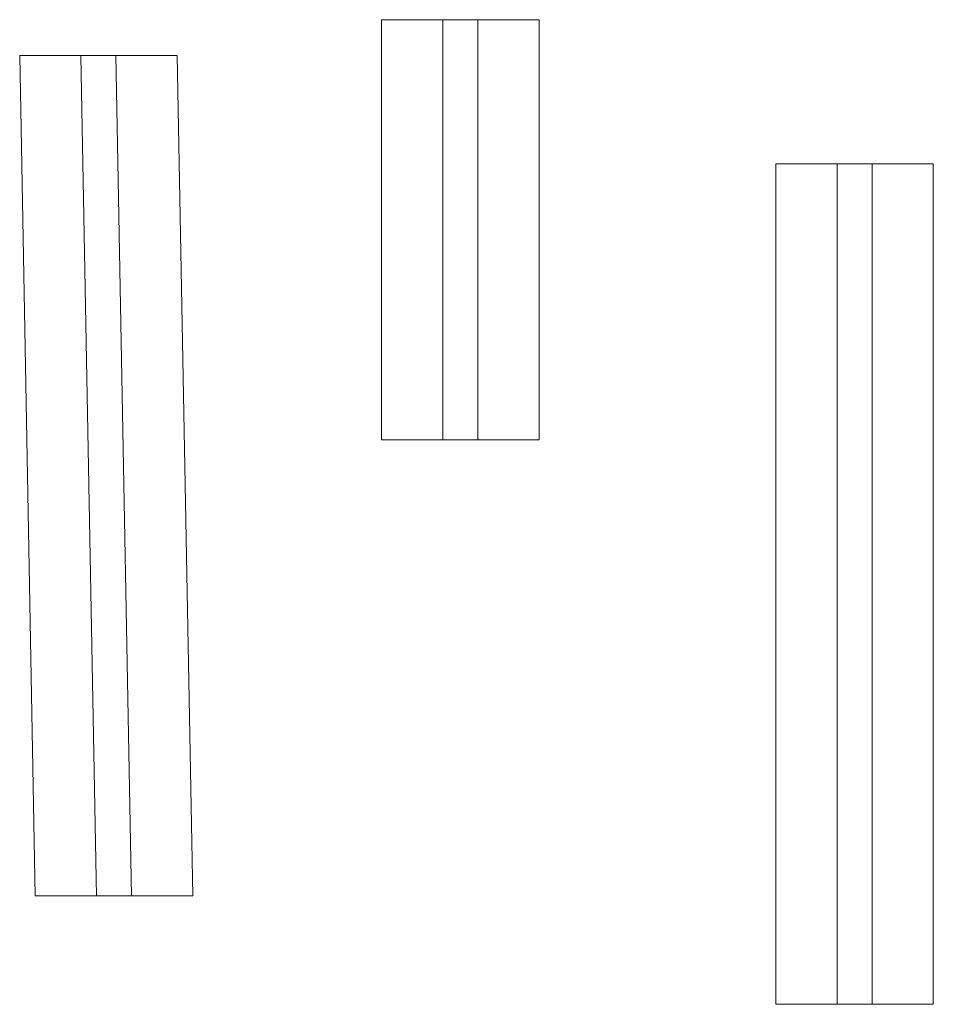
# Model space of a CAD drawing. Units: inches. Extents: x 292 to 2219, y -44 to 516.
# Tile 1 of 4: x 292 to 344, y 291 to 347. Entities that reach past the tile are written whole.
import ezdxf

# ---------------------------------------------------------------- set-up
doc = ezdxf.new("R2010")
doc.units = ezdxf.units.IN
doc.header["$MEASUREMENT"] = 0
doc.layers.add('A-GLAZ', color=34, linetype='Continuous', lineweight=18)

# ---------------------------------------------------------------- blocks, each defined once
blk = doc.blocks.new('WIN-48')
for p, q in [((0, 48), (9, 48)), ((0, 0), (0, 48)), ((3.5, 48), (3.5, 0)), ((5.5, 48), (5.5, 0)), ((9, 48), (9, 0)), ((9, 0), (0, 0))]:
    blk.add_line(p, q)
blk = doc.blocks.new('WIN-24')
for p, q in [((0, 24), (9, 24)), ((0, 24), (0, 0)), ((3.5, 24), (3.5, 0)), ((5.5, 24), (5.5, 0)), ((9, 24), (9, 0)), ((0, 0), (9, 0))]:
    blk.add_line(p, q)

msp = doc.modelspace()

# ---------------------------------------------------------------- linework, layer by layer
at = {"layer": 'A-GLAZ'}
for p, q in [((291.837, 345.031), (300.837, 345.031)), ((292.721, 297.039), (291.837, 345.031)), ((295.337, 345.012), (296.221, 297.02)), ((297.337, 345.049), (298.221, 297.057)), ((300.837, 345.031), (301.721, 297.039)), ((301.721, 297.039), (292.721, 297.039))]:
    msp.add_line(p, q, dxfattribs=at)

# ---------------------------------------------------------------- block references
for name, p in [('WIN-24', (312.51, 323.076)), ('WIN-48', (335.017, 290.838))]:
    msp.add_blockref(name, p, dxfattribs=at)

doc.saveas('drawing.dxf')
